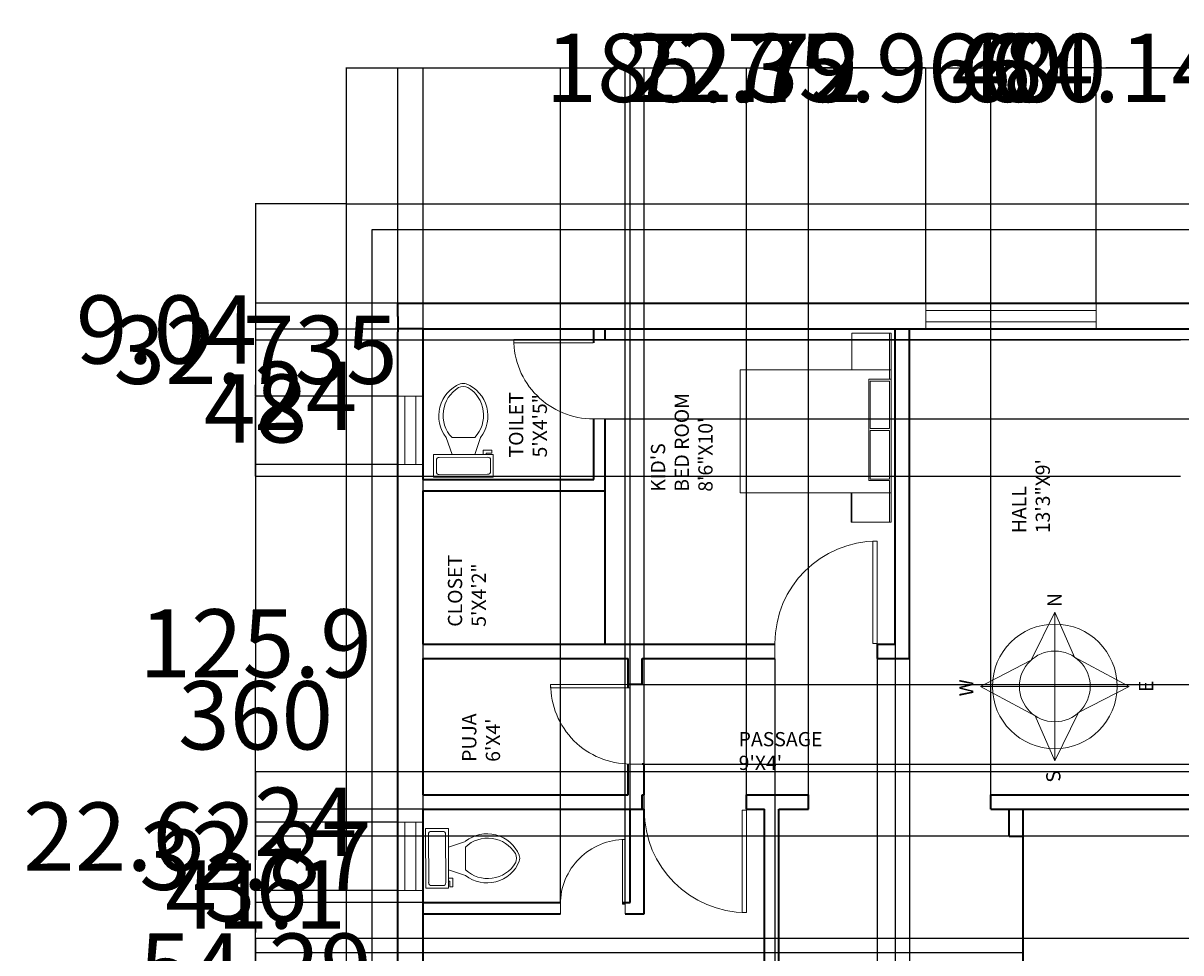
# Model space of a CAD drawing. Units: inches. Extents: x -1643 to -931, y 1907 to 2415.
# Tile 2 of 3: x -1643 to -1236, y 2088 to 2415. Entities that reach past the tile are written whole.
import ezdxf

# ---------------------------------------------------------------- set-up
doc = ezdxf.new("R2010")
doc.units = ezdxf.units.IN
for name, color, linetype, lineweight in [('A-ANNO-DIMS', 2, 'Continuous', 18), ('A-ANNO-SYMB', 7, 'Continuous', 18), ('A-AREA-IDEN', 7, 'Continuous', 18), ('A-DOOR', 3, 'Continuous', 18), ('A-FLOR-FIXT', 9, 'Continuous', 18), ('A-FURN', 8, 'Continuous', 18), ('A-GLAZ', 4, 'Continuous', 18), ('A-WALL', 7, 'Continuous', 35), ('C-PROP', 8, 'Continuous', 25)]:
    doc.layers.add(name, color=color, linetype=linetype, lineweight=lineweight)
doc.styles.get("Standard").update_dxf_attribs({"font": 'arial.ttf', "height": 24})
doc.dimstyles.get("Standard").update_dxf_attribs({"dimtxt": 0.18, "dimasz": 0.18, "dimexe": 0.18, "dimexo": 0.0625, "dimgap": 0.09, "dimtad": 0, "dimtih": 1, "dimtoh": 1, "dimdec": 4, "dimzin": 0, "dimdsep": 46, "dimtxsty": 'Standard', "dimcen": 0.09, "dimadec": 0, "dimazin": 0, "dimtfac": 1, "dimtdec": 4, "dimtofl": 0, "dimtmove": 0, "dimatfit": 3, "dimfxl": 1, "dimtolj": 1, "dimtzin": 0, "dimarcsym": 0})

# ---------------------------------------------------------------- blocks, each defined once
blk = doc.blocks.new('*U2')
for p, q in [((-40, 0), (-40, 6)), ((0, 0), (0, 6))]:
    blk.add_line(p, q)
blk.add_lwpolyline([(0, 0), (0, -40), (-1.75, -40), (-1.75, 0)], close=True)
blk.add_arc((0, 0), 40, 180, 270)
blk = doc.blocks.new('*U6')
for p, q in [((0, 0), (0, -6)), ((-40, 0), (-40, -6))]:
    blk.add_line(p, q)
blk.add_lwpolyline([(0, 0), (0, 40), (-1.75, 40), (-1.75, 0)], close=True)
blk.add_arc((0, 0), 40, 90, 180)
blk = doc.blocks.new('*U5')
for p, q in [((0, 0), (0, 6)), ((40, 0), (40, 6))]:
    blk.add_line(p, q)
blk.add_lwpolyline([(0, 0), (0, -40), (1.75, -40), (1.75, 0)], close=True)
blk.add_arc((0, 0), 40, 270, 0)
blk = doc.blocks.new('*U7')
for p, q in [((0, 5), (0, 0)), ((24, 5), (24, 0)), ((0, 2.5), (24, 2.5))]:
    blk.add_line(p, q)
blk = doc.blocks.new('*U10')
for p, q in [((0, 5), (0, 0)), ((60, 5), (60, 0)), ((0, 2.5), (60, 2.5))]:
    blk.add_line(p, q)
blk = doc.blocks.new('*U9')
for p, q in [((0, 5), (0, 0)), ((60, 5), (60, 0)), ((0, 2.5), (60, 2.5))]:
    blk.add_line(p, q)
blk = doc.blocks.new('*U15')
for p, q in [((-242, 177), (-242, 254)), ((-242, 254), (-216, 254)), ((-216, 254), (-216, 203)), ((-203, 101), (-356, 152)), ((-204, 177), (-242, 177)), ((-216, 203), (-204, 203)), ((-355, -102), (-356, 101)), ((-203, -102), (-355, -153)), ((-152, -242), (-50, -241))]:
    blk.add_line(p, q)
blk.add_lwpolyline([(-203, -267), (1, -267), (-1, 267), (-204, 266)], close=True)
for points in [[(-178, 216), (-177, -216)], [(-51, 241), (-153, 241)], [(-25, -216), (-26, 216)]]:
    blk.add_lwpolyline(points)
for centre, radius, start, end in [((-548, -90), 309, 51.5766, 158.079), ((-156, 219), 22.5, 81.9774, 188.2376), ((-48, 219), 22.5, 351.9774, 98.2376), ((-554, -108), 288, 46.4753, 149.0544), ((-737, -1), 102, 164.9681, 195.247), ((-708, -1), 102, 155.8394, 204.3757), ((-548, 88), 309, 202.136, 308.6382), ((-554, 106), 288, 211.1605, 313.7396), ((-155, -219), 22.5, 171.9774, 278.2376), ((-47, -219), 22.5, 261.9774, 8.2376)]:
    blk.add_arc(centre, radius, start, end)
blk = doc.blocks.new('BED-WITH-NIGHTSTANDS')
for p, q in [((10.33, 53.09), (53.66, 53.09)), ((10.33, 0.09), (10.33, 53.09)), ((53.66, 0.09), (53.66, 53.09)), ((0, 0), (0, 14.11)), ((0, 14.11), (10.33, 14.11)), ((0, 13.84), (10.33, 13.84)), ((53.66, 13.84), (66.5, 13.84)), ((66.5, 0.09), (66.5, 13.84)), ((14.66, 7.89), (50.39, 7.89)), ((14.66, 0.59), (14.66, 7.89)), ((15.11, 7.37), (32.28, 7.37)), ((15.11, 0.59), (15.11, 7.37)), ((32.28, 0.59), (32.28, 7.37)), ((33.01, 0.59), (33.01, 7.37)), ((33.01, 7.37), (49.65, 7.37)), ((49.65, 0.59), (49.65, 7.37)), ((50.39, 0.09), (50.39, 7.89)), ((0, 0.59), (14.66, 0.59)), ((0, 0.09), (66.5, 0.09)), ((15.11, 0.59), (32.28, 0.59)), ((33.01, 0.59), (49.65, 0.59)), ((50.39, 0.59), (66.5, 0.59))]:
    blk.add_line(p, q)
blk = doc.blocks.new('*D21')
at = {"layer": 'A-ANNO-DIMS', "color": 0, "lineweight": -2, "transparency": 16777216}
for p, q in [((-1529.17, 2351.21), (-1529.17, 2399.16)), ((-1528.99, 2398.98), (-1316.21, 2398.98)), ((-1049.35, 2398.98), (-1262.12, 2398.98)), ((-1049.17, 2351.21), (-1049.17, 2399.16))]:
    blk.add_line(p, q, dxfattribs=at)
at = {"layer": 'A-ANNO-DIMS', "color": 0, "transparency": 16777216}
for points in [[(-1528.99, 2399.01), (-1528.99, 2398.95), (-1529.17, 2398.98)], [(-1049.35, 2399.01), (-1049.35, 2398.95), (-1049.17, 2398.98)]]:
    blk.add_solid(points, dxfattribs=at)
at = {"layer": 'Defpoints', "color": 0, "transparency": 16777216}
for p in [(-1049.17, 2398.98), (-1529.17, 2351.15), (-1049.17, 2351.15)]:
    blk.add_point(p, dxfattribs=at)
at = {"layer": 'A-ANNO-DIMS', "color": 0, "transparency": 16777216, "insert": (-1289.17, 2398.98), "char_height": 24, "attachment_point": 5}
blk.add_mtext('\\A1;480', dxfattribs=at)
blk = doc.blocks.new('*D22')
at = {"layer": 'A-ANNO-DIMS', "color": 0, "lineweight": -2, "transparency": 16777216}
for p, q in [((-1529.23, 2351.15), (-1561.32, 2351.15)), ((-1561.14, 2350.97), (-1561.14, 2183.5)), ((-1561.14, 1991.33), (-1561.14, 2158.79)), ((-1529.23, 1991.15), (-1561.32, 1991.15))]:
    blk.add_line(p, q, dxfattribs=at)
at = {"layer": 'A-ANNO-DIMS', "color": 0, "transparency": 16777216}
for points in [[(-1561.17, 2350.97), (-1561.11, 2350.97), (-1561.14, 2351.15)], [(-1561.17, 1991.33), (-1561.11, 1991.33), (-1561.14, 1991.15)]]:
    blk.add_solid(points, dxfattribs=at)
at = {"layer": 'Defpoints', "color": 0, "transparency": 16777216}
for p in [(-1561.14, 2351.15), (-1529.17, 2351.15), (-1529.17, 1991.15)]:
    blk.add_point(p, dxfattribs=at)
at = {"layer": 'A-ANNO-DIMS', "color": 0, "transparency": 16777216, "insert": (-1561.14, 2171.15), "char_height": 24, "attachment_point": 5}
blk.add_mtext('\\A1;360', dxfattribs=at)
blk = doc.blocks.new('*D24')
at = {"layer": 'A-ANNO-DIMS', "color": 0, "lineweight": -2, "transparency": 16777216}
for p, q in [((-1511.17, 2316.21), (-1511.17, 2399.16)), ((-1510.99, 2398.98), (-1457.78, 2398.98)), ((-1325.66, 2398.98), (-1378.87, 2398.98)), ((-1325.48, 2316.19), (-1325.48, 2399.16))]:
    blk.add_line(p, q, dxfattribs=at)
at = {"layer": 'A-ANNO-DIMS', "color": 0, "transparency": 16777216}
for points in [[(-1510.99, 2399.01), (-1510.99, 2398.95), (-1511.17, 2398.98)], [(-1325.66, 2399.01), (-1325.66, 2398.95), (-1325.48, 2398.98)]]:
    blk.add_solid(points, dxfattribs=at)
at = {"layer": 'Defpoints', "color": 0, "transparency": 16777216}
for p in [(-1325.48, 2398.98), (-1511.17, 2316.15), (-1325.48, 2316.13)]:
    blk.add_point(p, dxfattribs=at)
at = {"layer": 'A-ANNO-DIMS', "color": 0, "transparency": 16777216, "insert": (-1418.32, 2398.98), "char_height": 24, "attachment_point": 5}
blk.add_mtext('\\A1;185.7', dxfattribs=at)
blk = doc.blocks.new('*D25')
at = {"layer": 'A-ANNO-DIMS', "color": 0, "lineweight": -2, "transparency": 16777216}
for p, q in [((-1325.48, 2316.19), (-1325.48, 2399.16)), ((-1325.3, 2398.98), (-1312.78, 2398.98)), ((-1265.66, 2398.98), (-1278.17, 2398.98)), ((-1265.48, 2316.19), (-1265.48, 2399.16))]:
    blk.add_line(p, q, dxfattribs=at)
at = {"layer": 'A-ANNO-DIMS', "color": 0, "transparency": 16777216}
for points in [[(-1325.3, 2399.01), (-1325.3, 2398.95), (-1325.48, 2398.98)], [(-1265.66, 2399.01), (-1265.66, 2398.95), (-1265.48, 2398.98)]]:
    blk.add_solid(points, dxfattribs=at)
at = {"layer": 'Defpoints', "color": 0, "transparency": 16777216}
for p in [(-1265.48, 2398.98), (-1325.48, 2316.13), (-1265.48, 2316.13)]:
    blk.add_point(p, dxfattribs=at)
at = {"layer": 'A-ANNO-DIMS', "color": 0, "transparency": 16777216, "insert": (-1295.48, 2398.98), "char_height": 24, "attachment_point": 5}
blk.add_mtext('\\A1;60', dxfattribs=at)
blk = doc.blocks.new('*D26')
at = {"layer": 'A-ANNO-DIMS', "color": 0, "lineweight": -2, "transparency": 16777216}
for p, q in [((-1265.48, 2316.19), (-1265.48, 2399.16)), ((-1265.3, 2398.98), (-1208.35, 2398.98)), ((-1208.17, 2316.21), (-1208.17, 2399.16)), ((-1208.17, 2398.98), (-1207.99, 2398.98))]:
    blk.add_line(p, q, dxfattribs=at)
at = {"layer": 'A-ANNO-DIMS', "color": 0, "transparency": 16777216}
for points in [[(-1265.3, 2399.01), (-1265.3, 2398.95), (-1265.48, 2398.98)], [(-1208.35, 2399.01), (-1208.35, 2398.95), (-1208.17, 2398.98)]]:
    blk.add_solid(points, dxfattribs=at)
at = {"layer": 'Defpoints', "color": 0, "transparency": 16777216}
for p in [(-1208.17, 2398.98), (-1265.48, 2316.13), (-1208.17, 2316.15)]:
    blk.add_point(p, dxfattribs=at)
at = {"layer": 'A-ANNO-DIMS', "color": 0, "transparency": 16777216, "insert": (-1169.72, 2398.98), "char_height": 24, "attachment_point": 5}
blk.add_mtext('\\A1;57.31', dxfattribs=at)
blk = doc.blocks.new('*D33')
at = {"layer": 'A-ANNO-DIMS', "color": 0, "lineweight": -2, "transparency": 16777216}
for p, q in [((-1502.23, 2138.15), (-1561.32, 2138.15)), ((-1561.14, 2137.97), (-1561.14, 2134.06)), ((-1561.14, 2105.46), (-1561.14, 2109.36)), ((-1502.23, 2105.28), (-1561.32, 2105.28))]:
    blk.add_line(p, q, dxfattribs=at)
at = {"layer": 'A-ANNO-DIMS', "color": 0, "transparency": 16777216}
for points in [[(-1561.17, 2137.97), (-1561.11, 2137.97), (-1561.14, 2138.15)], [(-1561.17, 2105.46), (-1561.11, 2105.46), (-1561.14, 2105.28)]]:
    blk.add_solid(points, dxfattribs=at)
at = {"layer": 'Defpoints', "color": 0, "transparency": 16777216}
for p in [(-1502.17, 2138.15), (-1561.14, 2105.28), (-1502.17, 2105.28)]:
    blk.add_point(p, dxfattribs=at)
at = {"layer": 'A-ANNO-DIMS', "color": 0, "transparency": 16777216, "insert": (-1561.14, 2121.71), "char_height": 24, "attachment_point": 5}
blk.add_mtext('\\A1;32.87', dxfattribs=at)
blk = doc.blocks.new('*D34')
at = {"layer": 'A-ANNO-DIMS', "color": 0, "lineweight": -2, "transparency": 16777216}
for p, q in [((-1502.17, 2138.21), (-1502.17, 2399.16)), ((-1501.99, 2398.98), (-1429.63, 2398.98)), ((-1429.45, 2138.21), (-1429.45, 2399.16)), ((-1429.45, 2398.98), (-1429.27, 2398.98))]:
    blk.add_line(p, q, dxfattribs=at)
at = {"layer": 'A-ANNO-DIMS', "color": 0, "transparency": 16777216}
for points in [[(-1501.99, 2399.01), (-1501.99, 2398.95), (-1502.17, 2398.98)], [(-1429.63, 2399.01), (-1429.63, 2398.95), (-1429.45, 2398.98)]]:
    blk.add_solid(points, dxfattribs=at)
at = {"layer": 'Defpoints', "color": 0, "transparency": 16777216}
for p in [(-1429.45, 2398.98), (-1502.17, 2138.15), (-1429.45, 2138.15)]:
    blk.add_point(p, dxfattribs=at)
at = {"layer": 'A-ANNO-DIMS', "color": 0, "transparency": 16777216, "insert": (-1388.91, 2398.98), "char_height": 24, "attachment_point": 5}
blk.add_mtext('\\A1;72.72', dxfattribs=at)
blk = doc.blocks.new('*D41')
at = {"layer": 'A-ANNO-DIMS', "color": 0, "lineweight": -2, "transparency": 16777216}
for p, q in [((-1235.81, 2303.15), (-1561.32, 2303.15)), ((-1561.14, 2302.97), (-1561.14, 2291.5)), ((-1561.14, 2255.33), (-1561.14, 2266.81)), ((-1235.81, 2255.15), (-1561.32, 2255.15))]:
    blk.add_line(p, q, dxfattribs=at)
at = {"layer": 'A-ANNO-DIMS', "color": 0, "transparency": 16777216}
for points in [[(-1561.17, 2302.97), (-1561.11, 2302.97), (-1561.14, 2303.15)], [(-1561.17, 2255.33), (-1561.11, 2255.33), (-1561.14, 2255.15)]]:
    blk.add_solid(points, dxfattribs=at)
at = {"layer": 'Defpoints', "color": 0, "transparency": 16777216}
for p in [(-1235.74, 2303.15), (-1561.14, 2255.15), (-1235.74, 2255.15)]:
    blk.add_point(p, dxfattribs=at)
at = {"layer": 'A-ANNO-DIMS', "color": 0, "transparency": 16777216, "insert": (-1561.14, 2279.15), "char_height": 24, "attachment_point": 5}
blk.add_mtext('\\A1;48', dxfattribs=at)
blk = doc.blocks.new('*D44')
at = {"layer": 'A-ANNO-DIMS', "color": 0, "lineweight": -2, "transparency": 16777216}
for p, q in [((-1213.24, 2151.26), (-1561.32, 2151.26)), ((-1561.14, 2151.08), (-1561.14, 2128.82)), ((-1213.11, 2128.64), (-1561.32, 2128.64)), ((-1561.14, 2128.46), (-1561.32, 2128.46)), ((-1561.14, 2128.64), (-1561.14, 2128.46))]:
    blk.add_line(p, q, dxfattribs=at)
at = {"layer": 'A-ANNO-DIMS', "color": 0, "transparency": 16777216}
for points in [[(-1561.17, 2151.08), (-1561.11, 2151.08), (-1561.14, 2151.26)], [(-1561.17, 2128.82), (-1561.11, 2128.82), (-1561.14, 2128.64)]]:
    blk.add_solid(points, dxfattribs=at)
at = {"layer": 'Defpoints', "color": 0, "transparency": 16777216}
for p in [(-1213.18, 2151.26), (-1561.14, 2128.64), (-1213.05, 2128.64)]:
    blk.add_point(p, dxfattribs=at)
at = {"layer": 'A-ANNO-DIMS', "color": 0, "transparency": 16777216, "insert": (-1601.99, 2128.46), "char_height": 24, "attachment_point": 5}
blk.add_mtext('\\A1;22.62', dxfattribs=at)
blk = doc.blocks.new('*D45')
at = {"layer": 'A-ANNO-DIMS', "color": 0, "lineweight": -2, "transparency": 16777216}
for p, q in [((-1213.11, 2128.64), (-1561.32, 2128.64)), ((-1561.14, 2128.46), (-1561.14, 2122.99)), ((-1561.14, 2092.82), (-1561.14, 2098.29)), ((-1213.11, 2092.64), (-1561.32, 2092.64))]:
    blk.add_line(p, q, dxfattribs=at)
at = {"layer": 'A-ANNO-DIMS', "color": 0, "transparency": 16777216}
for points in [[(-1561.17, 2128.46), (-1561.11, 2128.46), (-1561.14, 2128.64)], [(-1561.17, 2092.82), (-1561.11, 2092.82), (-1561.14, 2092.64)]]:
    blk.add_solid(points, dxfattribs=at)
at = {"layer": 'Defpoints', "color": 0, "transparency": 16777216}
for p in [(-1213.05, 2128.64), (-1561.14, 2092.64), (-1213.05, 2092.64)]:
    blk.add_point(p, dxfattribs=at)
at = {"layer": 'A-ANNO-DIMS', "color": 0, "transparency": 16777216, "insert": (-1561.14, 2110.64), "char_height": 24, "attachment_point": 5}
blk.add_mtext('\\A1;36', dxfattribs=at)
blk = doc.blocks.new('*D46')
at = {"layer": 'A-ANNO-DIMS', "color": 0, "lineweight": -2, "transparency": 16777216}
for p, q in [((-1213.11, 2092.64), (-1561.32, 2092.64)), ((-1561.14, 2092.46), (-1561.14, 2067.69)), ((-1561.14, 2018.33), (-1561.14, 2043.1)), ((-1213.23, 2018.15), (-1561.32, 2018.15))]:
    blk.add_line(p, q, dxfattribs=at)
at = {"layer": 'A-ANNO-DIMS', "color": 0, "transparency": 16777216}
for points in [[(-1561.17, 2092.46), (-1561.11, 2092.46), (-1561.14, 2092.64)], [(-1561.17, 2018.33), (-1561.11, 2018.33), (-1561.14, 2018.15)]]:
    blk.add_solid(points, dxfattribs=at)
at = {"layer": 'Defpoints', "color": 0, "transparency": 16777216}
for p in [(-1213.05, 2092.64), (-1561.14, 2018.15), (-1213.17, 2018.15)]:
    blk.add_point(p, dxfattribs=at)
at = {"layer": 'A-ANNO-DIMS', "color": 0, "transparency": 16777216, "insert": (-1561.14, 2055.39), "char_height": 24, "attachment_point": 5}
blk.add_mtext('\\A1;74.5', dxfattribs=at)
blk = doc.blocks.new('*D49')
at = {"layer": 'A-ANNO-DIMS', "color": 0, "lineweight": -2, "transparency": 16777216}
for p, q in [((-1511.21, 2109.52), (-1561.32, 2109.52)), ((-1561.14, 2109.34), (-1561.14, 2094.71)), ((-1561.14, 2055.4), (-1561.14, 2070.03)), ((-1511.27, 2055.22), (-1561.32, 2055.22))]:
    blk.add_line(p, q, dxfattribs=at)
at = {"layer": 'A-ANNO-DIMS', "color": 0, "transparency": 16777216}
for points in [[(-1561.17, 2109.34), (-1561.11, 2109.34), (-1561.14, 2109.52)], [(-1561.17, 2055.4), (-1561.11, 2055.4), (-1561.14, 2055.22)]]:
    blk.add_solid(points, dxfattribs=at)
at = {"layer": 'Defpoints', "color": 0, "transparency": 16777216}
for p in [(-1561.14, 2109.52), (-1511.15, 2109.52), (-1511.21, 2055.22)]:
    blk.add_point(p, dxfattribs=at)
at = {"layer": 'A-ANNO-DIMS', "color": 0, "transparency": 16777216, "insert": (-1561.14, 2082.37), "char_height": 24, "attachment_point": 5}
blk.add_mtext('\\A1;54.29', dxfattribs=at)
blk = doc.blocks.new('*D50')
at = {"layer": 'A-ANNO-DIMS', "color": 0, "lineweight": -2, "transparency": 16777216}
for p, q in [((-1511.21, 2133.52), (-1561.32, 2133.52)), ((-1561.14, 2133.52), (-1561.14, 2133.7)), ((-1561.14, 2133.7), (-1560.96, 2133.7)), ((-1561.14, 2109.7), (-1561.14, 2133.34)), ((-1511.21, 2109.52), (-1561.32, 2109.52))]:
    blk.add_line(p, q, dxfattribs=at)
at = {"layer": 'A-ANNO-DIMS', "color": 0, "transparency": 16777216}
for points in [[(-1561.17, 2133.34), (-1561.11, 2133.34), (-1561.14, 2133.52)], [(-1561.17, 2109.7), (-1561.11, 2109.7), (-1561.14, 2109.52)]]:
    blk.add_solid(points, dxfattribs=at)
at = {"layer": 'Defpoints', "color": 0, "transparency": 16777216}
for p in [(-1561.14, 2133.52), (-1511.15, 2133.52), (-1511.15, 2109.52)]:
    blk.add_point(p, dxfattribs=at)
at = {"layer": 'A-ANNO-DIMS', "color": 0, "transparency": 16777216, "insert": (-1543.53, 2133.7), "char_height": 24, "attachment_point": 5}
blk.add_mtext('\\A1;24', dxfattribs=at)
blk = doc.blocks.new('*D51')
at = {"layer": 'A-ANNO-DIMS', "color": 0, "lineweight": -2, "transparency": 16777216}
for p, q in [((-1511.22, 2259.41), (-1561.32, 2259.41)), ((-1561.14, 2259.23), (-1561.14, 2208.81)), ((-1561.14, 2133.7), (-1561.14, 2184.12)), ((-1511.21, 2133.52), (-1561.32, 2133.52))]:
    blk.add_line(p, q, dxfattribs=at)
at = {"layer": 'A-ANNO-DIMS', "color": 0, "transparency": 16777216}
for points in [[(-1561.17, 2259.23), (-1561.11, 2259.23), (-1561.14, 2259.41)], [(-1561.17, 2133.7), (-1561.11, 2133.7), (-1561.14, 2133.52)]]:
    blk.add_solid(points, dxfattribs=at)
at = {"layer": 'Defpoints', "color": 0, "transparency": 16777216}
for p in [(-1561.14, 2259.41), (-1511.16, 2259.41), (-1511.15, 2133.52)]:
    blk.add_point(p, dxfattribs=at)
at = {"layer": 'A-ANNO-DIMS', "color": 0, "transparency": 16777216, "insert": (-1561.14, 2196.46), "char_height": 24, "attachment_point": 5}
blk.add_mtext('\\A1;125.9', dxfattribs=at)
blk = doc.blocks.new('*D52')
at = {"layer": 'A-ANNO-DIMS', "color": 0, "lineweight": -2, "transparency": 16777216}
for p, q in [((-1511.22, 2283.41), (-1561.32, 2283.41)), ((-1561.14, 2283.41), (-1561.14, 2283.59)), ((-1561.14, 2283.59), (-1560.96, 2283.59)), ((-1561.14, 2259.59), (-1561.14, 2283.23)), ((-1511.22, 2259.41), (-1561.32, 2259.41))]:
    blk.add_line(p, q, dxfattribs=at)
at = {"layer": 'A-ANNO-DIMS', "color": 0, "transparency": 16777216}
for points in [[(-1561.17, 2283.23), (-1561.11, 2283.23), (-1561.14, 2283.41)], [(-1561.17, 2259.59), (-1561.11, 2259.59), (-1561.14, 2259.41)]]:
    blk.add_solid(points, dxfattribs=at)
at = {"layer": 'Defpoints', "color": 0, "transparency": 16777216}
for p in [(-1561.14, 2283.41), (-1511.16, 2283.41), (-1511.16, 2259.41)]:
    blk.add_point(p, dxfattribs=at)
at = {"layer": 'A-ANNO-DIMS', "color": 0, "transparency": 16777216, "insert": (-1543.53, 2283.59), "char_height": 24, "attachment_point": 5}
blk.add_mtext('\\A1;24', dxfattribs=at)
blk = doc.blocks.new('*D53')
at = {"layer": 'A-ANNO-DIMS', "color": 0, "lineweight": -2, "transparency": 16777216}
for p, q in [((-1511.23, 2316.15), (-1561.32, 2316.15)), ((-1561.14, 2315.97), (-1561.14, 2312.13)), ((-1561.14, 2283.59), (-1561.14, 2287.43)), ((-1511.22, 2283.41), (-1561.32, 2283.41))]:
    blk.add_line(p, q, dxfattribs=at)
at = {"layer": 'A-ANNO-DIMS', "color": 0, "transparency": 16777216}
for points in [[(-1561.17, 2315.97), (-1561.11, 2315.97), (-1561.14, 2316.15)], [(-1561.17, 2283.59), (-1561.11, 2283.59), (-1561.14, 2283.41)]]:
    blk.add_solid(points, dxfattribs=at)
at = {"layer": 'Defpoints', "color": 0, "transparency": 16777216}
for p in [(-1561.14, 2316.15), (-1511.17, 2316.15), (-1511.16, 2283.41)]:
    blk.add_point(p, dxfattribs=at)
at = {"layer": 'A-ANNO-DIMS', "color": 0, "transparency": 16777216, "insert": (-1561.14, 2299.78), "char_height": 24, "attachment_point": 5}
blk.add_mtext('\\A1;32.735', dxfattribs=at)
blk = doc.blocks.new('*D54')
at = {"layer": 'A-ANNO-DIMS', "color": 0, "lineweight": -2, "transparency": 16777216}
for p, q in [((-1438.11, 2303.44), (-971.69, 2303.44)), ((-971.87, 2303.26), (-971.87, 2301.79)), ((-971.87, 2275.62), (-971.87, 2277.1)), ((-1438.11, 2275.44), (-971.69, 2275.44))]:
    blk.add_line(p, q, dxfattribs=at)
at = {"layer": 'A-ANNO-DIMS', "color": 0, "transparency": 16777216}
for points in [[(-971.9, 2303.26), (-971.84, 2303.26), (-971.87, 2303.44)], [(-971.9, 2275.62), (-971.84, 2275.62), (-971.87, 2275.44)]]:
    blk.add_solid(points, dxfattribs=at)
at = {"layer": 'Defpoints', "color": 0, "transparency": 16777216}
for p in [(-1438.17, 2303.44), (-1438.17, 2275.44), (-971.87, 2275.44)]:
    blk.add_point(p, dxfattribs=at)
at = {"layer": 'A-ANNO-DIMS', "color": 0, "transparency": 16777216, "insert": (-971.87, 2289.44), "char_height": 24, "attachment_point": 5}
blk.add_mtext('\\A1;28', dxfattribs=at)
blk = doc.blocks.new('*D55')
at = {"layer": 'A-ANNO-DIMS', "color": 0, "lineweight": -2, "transparency": 16777216}
for p, q in [((-1378.5, 2191.08), (-1378.5, 1922.66)), ((-1342.5, 2191.08), (-1342.5, 1922.66)), ((-1378.32, 1922.84), (-1377.76, 1922.84)), ((-1342.68, 1922.84), (-1343.23, 1922.84))]:
    blk.add_line(p, q, dxfattribs=at)
at = {"layer": 'A-ANNO-DIMS', "color": 0, "transparency": 16777216}
for points in [[(-1378.32, 1922.87), (-1378.32, 1922.81), (-1378.5, 1922.84)], [(-1342.68, 1922.87), (-1342.68, 1922.81), (-1342.5, 1922.84)]]:
    blk.add_solid(points, dxfattribs=at)
at = {"layer": 'Defpoints', "color": 0, "transparency": 16777216}
for p in [(-1378.5, 2191.15), (-1342.5, 2191.15), (-1342.5, 1922.84)]:
    blk.add_point(p, dxfattribs=at)
at = {"layer": 'A-ANNO-DIMS', "color": 0, "transparency": 16777216, "insert": (-1360.5, 1922.84), "char_height": 24, "attachment_point": 5}
blk.add_mtext('\\A1;36', dxfattribs=at)
blk = doc.blocks.new('*D56')
at = {"layer": 'A-ANNO-DIMS', "color": 0, "lineweight": -2, "transparency": 16777216}
for p, q in [((-1425.11, 2182), (-971.69, 2182)), ((-971.87, 2181.82), (-971.87, 2180.35)), ((-1424.39, 2154), (-971.69, 2154)), ((-971.87, 2154.18), (-971.87, 2155.66))]:
    blk.add_line(p, q, dxfattribs=at)
at = {"layer": 'A-ANNO-DIMS', "color": 0, "transparency": 16777216}
for points in [[(-971.9, 2181.82), (-971.84, 2181.82), (-971.87, 2182)], [(-971.9, 2154.18), (-971.84, 2154.18), (-971.87, 2154)]]:
    blk.add_solid(points, dxfattribs=at)
at = {"layer": 'Defpoints', "color": 0, "transparency": 16777216}
for p in [(-1425.17, 2182), (-1424.45, 2154), (-971.87, 2154)]:
    blk.add_point(p, dxfattribs=at)
at = {"layer": 'A-ANNO-DIMS', "color": 0, "transparency": 16777216, "insert": (-971.87, 2168), "char_height": 24, "attachment_point": 5}
blk.add_mtext('\\A1;28', dxfattribs=at)
blk = doc.blocks.new('*D57')
at = {"layer": 'A-ANNO-DIMS', "color": 0, "lineweight": -2, "transparency": 16777216}
for p, q in [((-1424.45, 2138.21), (-1424.45, 2399.16)), ((-1424.27, 2398.98), (-1388.66, 2398.98)), ((-1388.48, 2138.21), (-1388.48, 2399.16)), ((-1388.48, 2398.98), (-1388.3, 2398.98))]:
    blk.add_line(p, q, dxfattribs=at)
at = {"layer": 'A-ANNO-DIMS', "color": 0, "transparency": 16777216}
for points in [[(-1424.27, 2399.01), (-1424.27, 2398.95), (-1424.45, 2398.98)], [(-1388.66, 2399.01), (-1388.66, 2398.95), (-1388.48, 2398.98)]]:
    blk.add_solid(points, dxfattribs=at)
at = {"layer": 'Defpoints', "color": 0, "transparency": 16777216}
for p in [(-1388.48, 2398.98), (-1424.45, 2138.15), (-1388.48, 2138.15)]:
    blk.add_point(p, dxfattribs=at)
at = {"layer": 'A-ANNO-DIMS', "color": 0, "transparency": 16777216, "insert": (-1338.41, 2398.98), "char_height": 24, "attachment_point": 5}
blk.add_mtext('\\A1;35.966', dxfattribs=at)
blk = doc.blocks.new('*D58')
at = {"layer": 'A-ANNO-DIMS', "color": 0, "lineweight": -2, "transparency": 16777216}
for p, q in [((-1453.94, 2105.34), (-1453.94, 2399.16)), ((-1453.76, 2398.98), (-1431.33, 2398.98)), ((-1431.15, 2104.72), (-1431.15, 2399.16)), ((-1431.15, 2398.98), (-1430.97, 2398.98))]:
    blk.add_line(p, q, dxfattribs=at)
at = {"layer": 'A-ANNO-DIMS', "color": 0, "transparency": 16777216}
for points in [[(-1453.76, 2399.01), (-1453.76, 2398.95), (-1453.94, 2398.98)], [(-1431.33, 2399.01), (-1431.33, 2398.95), (-1431.15, 2398.98)]]:
    blk.add_solid(points, dxfattribs=at)
at = {"layer": 'Defpoints', "color": 0, "transparency": 16777216}
for p in [(-1431.15, 2398.98), (-1453.94, 2105.28), (-1431.15, 2104.65)]:
    blk.add_point(p, dxfattribs=at)
at = {"layer": 'A-ANNO-DIMS', "color": 0, "transparency": 16777216, "insert": (-1390.16, 2398.98), "char_height": 24, "attachment_point": 5}
blk.add_mtext('\\A1;22.79', dxfattribs=at)
blk = doc.blocks.new('*D59')
at = {"layer": 'A-ANNO-DIMS', "color": 0, "lineweight": -2, "transparency": 16777216}
for p, q in [((-1366.66, 2143.21), (-1366.66, 2399.16)), ((-1366.48, 2398.98), (-1302.71, 2398.98)), ((-1302.53, 2143.21), (-1302.53, 2399.16)), ((-1302.53, 2398.98), (-1302.35, 2398.98))]:
    blk.add_line(p, q, dxfattribs=at)
at = {"layer": 'A-ANNO-DIMS', "color": 0, "transparency": 16777216}
for points in [[(-1366.48, 2399.01), (-1366.48, 2398.95), (-1366.66, 2398.98)], [(-1302.71, 2399.01), (-1302.71, 2398.95), (-1302.53, 2398.98)]]:
    blk.add_solid(points, dxfattribs=at)
at = {"layer": 'Defpoints', "color": 0, "transparency": 16777216}
for p in [(-1302.53, 2398.98), (-1366.66, 2143.15), (-1302.53, 2143.15)]:
    blk.add_point(p, dxfattribs=at)
at = {"layer": 'A-ANNO-DIMS', "color": 0, "transparency": 16777216, "insert": (-1261.75, 2398.98), "char_height": 24, "attachment_point": 5}
blk.add_mtext('\\A1;64.14', dxfattribs=at)
blk = doc.blocks.new('*D60')
at = {"layer": 'A-ANNO-DIMS', "color": 0, "lineweight": -2, "transparency": 16777216}
for p, q in [((-1291.23, 2128.66), (-1561.32, 2128.66)), ((-1561.14, 2128.48), (-1561.14, 2120.24)), ((-1561.14, 2087.74), (-1561.14, 2095.97)), ((-1291.23, 2087.56), (-1561.32, 2087.56))]:
    blk.add_line(p, q, dxfattribs=at)
at = {"layer": 'A-ANNO-DIMS', "color": 0, "transparency": 16777216}
for points in [[(-1561.17, 2128.48), (-1561.11, 2128.48), (-1561.14, 2128.66)], [(-1561.17, 2087.74), (-1561.11, 2087.74), (-1561.14, 2087.56)]]:
    blk.add_solid(points, dxfattribs=at)
at = {"layer": 'Defpoints', "color": 0, "transparency": 16777216}
for p in [(-1561.14, 2128.66), (-1291.17, 2128.66), (-1291.17, 2087.56)]:
    blk.add_point(p, dxfattribs=at)
at = {"layer": 'A-ANNO-DIMS', "color": 0, "transparency": 16777216, "insert": (-1561.14, 2108.11), "char_height": 24, "attachment_point": 5}
blk.add_mtext('\\A1;41.1', dxfattribs=at)
blk = doc.blocks.new('*D61')
at = {"layer": 'A-ANNO-DIMS', "color": 0, "lineweight": -2, "transparency": 16777216}
for p, q in [((-1325.54, 2316.13), (-1561.32, 2316.13)), ((-1561.14, 2315.95), (-1561.14, 2307.27)), ((-1325.54, 2307.09), (-1561.32, 2307.09)), ((-1561.14, 2306.91), (-1561.32, 2306.91)), ((-1561.14, 2307.09), (-1561.14, 2306.91))]:
    blk.add_line(p, q, dxfattribs=at)
at = {"layer": 'A-ANNO-DIMS', "color": 0, "transparency": 16777216}
for points in [[(-1561.17, 2315.95), (-1561.11, 2315.95), (-1561.14, 2316.13)], [(-1561.17, 2307.27), (-1561.11, 2307.27), (-1561.14, 2307.09)]]:
    blk.add_solid(points, dxfattribs=at)
at = {"layer": 'Defpoints', "color": 0, "transparency": 16777216}
for p in [(-1325.48, 2316.13), (-1561.14, 2307.09), (-1325.48, 2307.09)]:
    blk.add_point(p, dxfattribs=at)
at = {"layer": 'A-ANNO-DIMS', "color": 0, "transparency": 16777216, "insert": (-1592.53, 2306.91), "char_height": 24, "attachment_point": 5}
blk.add_mtext('\\A1;9.04', dxfattribs=at)
blk = doc.blocks.new('*D62')
at = {"layer": 'A-ANNO-DIMS', "color": 0, "lineweight": -2, "transparency": 16777216}
for p, q in [((-1336.17, 2196.08), (-1336.17, 1922.66)), ((-1331.15, 2191.08), (-1331.15, 1922.66)), ((-1335.99, 1922.84), (-1331.33, 1922.84)), ((-1331.15, 1922.84), (-1330.97, 1922.84))]:
    blk.add_line(p, q, dxfattribs=at)
at = {"layer": 'A-ANNO-DIMS', "color": 0, "transparency": 16777216}
for points in [[(-1335.99, 1922.87), (-1335.99, 1922.81), (-1336.17, 1922.84)], [(-1331.33, 1922.87), (-1331.33, 1922.81), (-1331.15, 1922.84)]]:
    blk.add_solid(points, dxfattribs=at)
at = {"layer": 'Defpoints', "color": 0, "transparency": 16777216}
for p in [(-1336.17, 2196.15), (-1331.15, 2191.15), (-1331.15, 1922.84)]:
    blk.add_point(p, dxfattribs=at)
at = {"layer": 'A-ANNO-DIMS', "color": 0, "transparency": 16777216, "insert": (-1290.39, 1922.84), "char_height": 24, "attachment_point": 5}
blk.add_mtext('\\A1;5.013', dxfattribs=at)

msp = doc.modelspace()

# ---------------------------------------------------------------- linework, layer by layer
at = {"layer": 'A-ANNO-SYMB'}
for p, q in [((-1288.4285, 2190.5496), (-1280.072, 2207.4636)), ((-1280.072, 2207.4636), (-1273.1474, 2191.6673)), ((-1280.072, 2155.1759), (-1280.072, 2207.4636)), ((-1288.4285, 2190.5496), (-1306.2158, 2181.3197)), ((-1253.9281, 2181.3197), (-1273.1474, 2191.6673)), ((-1306.2158, 2181.3197), (-1286.9965, 2170.9721)), ((-1306.2158, 2181.3197), (-1253.9281, 2181.3197)), ((-1280.072, 2181.3197), (-1280.072, 2181.3197)), ((-1271.7154, 2172.0899), (-1253.9281, 2181.3197)), ((-1286.9965, 2170.9721), (-1280.072, 2155.1759)), ((-1280.072, 2155.1759), (-1271.7154, 2172.0899))]:
    msp.add_line(p, q, dxfattribs=at)
for radius in [21.9386, 12.4508]:
    msp.add_circle((-1280.072, 2181.3197), radius, dxfattribs=at)
at = {"layer": 'A-WALL'}
for p, q in [((-1511.1668, 2316.1464), (-1131.1668, 2316.1464)), ((-1511.1668, 2311.4873), (-1511.1668, 2316.1464)), ((-1511.1668, 2311.4873), (-1511.1668, 2306.1464)), ((-1502.1668, 2307.1464), (-1511.1668, 2307.1464)), ((-1511.1668, 2009.1464), (-1511.1668, 2306.1464)), ((-1502.1668, 2306.1464), (-1502.1668, 2307.1464)), ((-1502.1668, 2307.1464), (-1213.1668, 2307.1464)), ((-1502.1668, 2254.1464), (-1502.1668, 2306.1464)), ((-1442.1668, 2306.1464), (-1442.1668, 2307.1464)), ((-1442.1668, 2302.2175), (-1442.1668, 2306.1464)), ((-1438.1668, 2306.1464), (-1438.1668, 2307.1464)), ((-1438.1668, 2303.4425), (-1438.1668, 2306.1464)), ((-1336.1668, 2306.1464), (-1336.1668, 2307.1464)), ((-1336.1668, 2196.1464), (-1336.1668, 2306.1464)), ((-1331.1668, 2306.1464), (-1331.1668, 2307.1464)), ((-1331.1668, 2196.1464), (-1331.1668, 2306.1464)), ((-1442.1668, 2254.1464), (-1442.1668, 2275.4654)), ((-1438.1668, 2196.1464), (-1438.1668, 2275.4425)), ((-1502.1668, 2254.1464), (-1442.1668, 2254.1464)), ((-1502.1668, 2250.1464), (-1438.1668, 2250.1464)), ((-1502.1668, 2196.1464), (-1502.1668, 2250.1464)), ((-1502.1668, 2196.1464), (-1378.4982, 2196.1464)), ((-1342.4982, 2196.1464), (-1336.1668, 2196.1464)), ((-1342.4982, 2196.1464), (-1342.4982, 2191.1464)), ((-1331.1542, 2191.1464), (-1331.1668, 2196.1464)), ((-1502.1668, 2191.1464), (-1430.1668, 2191.1464)), ((-1502.1668, 2143.1464), (-1502.1668, 2191.1464)), ((-1430.1668, 2180.7784), (-1430.1668, 2191.1464)), ((-1425.1668, 2191.1464), (-1378.4982, 2191.1464)), ((-1425.1668, 2182.1464), (-1425.1668, 2191.1464)), ((-1342.4982, 2191.1464), (-1331.1542, 2191.1464)), ((-1430.1668, 2182.1464), (-1425.1668, 2182.1464)), ((-1430.1668, 2143.1464), (-1430.1668, 2154.0147)), ((-1424.4498, 2154.0034), (-1425.1708, 2154.0034)), ((-1424.4498, 2143.1464), (-1424.4498, 2154.0034)), ((-1502.1668, 2143.1464), (-1430.1668, 2143.1464)), ((-1425.1668, 2138.1464), (-1425.1668, 2143.1464)), ((-1425.1668, 2143.1464), (-1424.4498, 2143.1464)), ((-1388.4842, 2138.1464), (-1388.4842, 2143.1464)), ((-1388.4842, 2143.1464), (-1382.1668, 2143.1464)), ((-1382.1668, 2143.1464), (-1366.6634, 2143.1464)), ((-1366.6634, 2138.1464), (-1366.6634, 2143.1464)), ((-1302.5278, 2143.1464), (-1213.1668, 2143.1464)), ((-1302.5278, 2138.1464), (-1302.5278, 2143.1464)), ((-1502.1668, 2018.1464), (-1502.1668, 2138.1464)), ((-1502.1668, 2138.1464), (-1425.1668, 2138.1464)), ((-1429.4498, 2105.2782), (-1429.4498, 2138.1464)), ((-1425.1668, 2138.1464), (-1424.4498, 2138.1464)), ((-1424.4498, 2101.2782), (-1424.4498, 2138.1464)), ((-1388.4842, 2138.1464), (-1382.1668, 2138.1464)), ((-1382.1668, 2018.1464), (-1382.1668, 2138.1464)), ((-1377.1668, 2018.1464), (-1377.1668, 2138.1464)), ((-1377.1668, 2138.1464), (-1366.6634, 2138.1464)), ((-1302.5278, 2138.1464), (-1296.1668, 2138.1464)), ((-1296.1668, 2138.1464), (-1291.1668, 2138.1464)), ((-1296.1668, 2138.1464), (-1291.1668, 2138.1464)), ((-1296.1668, 2128.6553), (-1296.1668, 2138.1464)), ((-1291.1668, 2018.1464), (-1291.1668, 2138.1464)), ((-1291.1668, 2138.1464), (-1213.1668, 2138.1464)), ((-1296.1668, 2128.6553), (-1291.1668, 2128.6553)), ((-1502.1668, 2105.2782), (-1453.9433, 2105.2782)), ((-1432.149, 2105.2782), (-1429.4498, 2105.2782)), ((-1502.1668, 2101.2782), (-1453.9519, 2101.2782)), ((-1431.1514, 2101.2782), (-1425.1668, 2101.2782)), ((-1425.1668, 2101.2782), (-1424.4498, 2101.2782))]:
    msp.add_line(p, q, dxfattribs=at)
at = {"layer": 'C-PROP'}
for p, q in [((-1529.1668, 1991.1464), (-1529.1668, 2351.1464)), ((-1529.1668, 2351.1464), (-1049.1668, 2351.1464)), ((-1520.1668, 2000.1464), (-1520.1668, 2342.1464)), ((-1520.1668, 2342.1464), (-1058.1668, 2342.1464))]:
    msp.add_line(p, q, dxfattribs=at)

# ---------------------------------------------------------------- block references
at = {"layer": 'A-DOOR'}
for p, xscale, yscale, zscale, rotation in [((-1442.3708, 2303.4425), 0.7000000000000001, 0.7000000000000001, 0.7000000000000001, 270), ((-1429.3708, 2182.0034), 0.7000000000000001, 0.7000000000000001, 0.7000000000000001, 270), ((-1431.1514, 2104.6534), 0.5700110980006006, 0.5700110980006006, 0.5700110980006006, 180)]:
    msp.add_blockref('*U5', p, dxfattribs=dict(at, xscale=xscale, yscale=yscale, zscale=zscale, rotation=rotation))
at = {"layer": 'A-DOOR', "xscale": 0.9, "yscale": 0.9, "zscale": 0.9}
for name, p in [('*U6', (-1342.4982, 2196.4667)), ('*U2', (-1388.4498, 2137.7465))]:
    msp.add_blockref(name, p, dxfattribs=at)
at = {"layer": 'A-FLOR-FIXT', "xscale": 0.0393700787401575, "yscale": 0.0393700787401575, "zscale": 0.0393700787401575}
for p, rotation in [((-1488.0437, 2254.9428), 270), ((-1501.2909, 2120.7761), 180)]:
    msp.add_blockref('*U15', p, dxfattribs=dict(at, rotation=rotation))
at = {"layer": 'A-FURN', "rotation": 90.0000000000013}
msp.add_blockref('BED-WITH-NIGHTSTANDS', (-1337.5769, 2239.0844), dxfattribs=at)
at = {"layer": 'A-GLAZ'}
for name, p in [('*U9', (-1325.4771, 2311.1314)), ('*U10', (-1325.478, 2307.092))]:
    msp.add_blockref(name, p, dxfattribs=at)
at = {"layer": 'A-GLAZ', "rotation": 270}
for p in [(-1511.1597, 2283.4112), (-1507.2375, 2283.4165), (-1511.1453, 2133.516), (-1507.2375, 2133.5243)]:
    msp.add_blockref('*U7', p, dxfattribs=at)

# ---------------------------------------------------------------- texts
at = {"layer": 'A-ANNO-SYMB', "char_height": 5, "attachment_point": 1}
for s, width, insert, rotation in [('N', 10.988887, (-1282.6739, 2209.2546), 90), ('W', 48.389659, (-1313.6974, 2177.8217), 90), ('E', 11.952828, (-1250.4755, 2179.3488), 90), ('S', 34.508966, (-1282.7555, 2147.2289), 98.36296)]:
    msp.add_mtext_dynamic_manual_height_columns(s, width=width, gutter_width=120, heights=[0], dxfattribs=dict(at, insert=insert, rotation=rotation))
at = {"layer": 'A-AREA-IDEN', "char_height": 5, "attachment_point": 1, "rotation": 90}
for s, width, insert in [('TOILET\\P5\'X4\'5"', 106.496123, (-1472.0099, 2261.8962)), ('KID\'S\\PBED ROOM\\P8\'6"X10\'', 50.968561, (-1422.0953, 2249.8293)), ('HALL\\P13\'3"X9\'', 56.726574, (-1295.1218, 2235.2391)), ('CLOSET\\P5\'X4\'2"', 73.534199, (-1493.4986, 2202.3169)), ("PUJA\\P6'X4'", 153.656396, (-1488.4992, 2154.7803))]:
    msp.add_mtext_dynamic_manual_height_columns(s, width=width, gutter_width=120, heights=[0], dxfattribs=dict(at, insert=insert))
at = {"layer": 'A-AREA-IDEN', "insert": (-1391.2395, 2165.256), "char_height": 5, "attachment_point": 1}
msp.add_mtext_dynamic_manual_height_columns("PASSAGE\\P9'X4'", width=49.293418, gutter_width=120, heights=[0], dxfattribs=at)

# ---------------------------------------------------------------- dimensions: what is measured, and where the dimension line sits
at = {"layer": 'A-ANNO-DIMS'}
for base, p1, p2, override, picture, middle in [((-1049.1668, 2398.9832), (-1529.1668, 2351.1464), (-1049.1668, 2351.1464), {"dimdec": 0, "dimlfac": 1, "dimrnd": 0, "dimzin": 0, "dimdsep": 46, "dimlunit": 2}, '*D21', (-1289.1668, 2398.9832)), ((-1325.4771, 2398.9832), (-1511.1668, 2316.1464), (-1325.4771, 2316.1314), {"dimdec": 1, "dimlfac": 1, "dimrnd": 0, "dimzin": 0, "dimdsep": 46, "dimlunit": 2}, '*D24', (-1418.322, 2398.9832)), ((-1429.4498, 2398.9832), (-1502.1668, 2138.1464), (-1429.4498, 2138.1464), {"dimdec": 2, "dimlfac": 1, "dimrnd": 0, "dimzin": 0, "dimdsep": 46, "dimlunit": 2}, '*D34', (-1388.9069, 2398.9832)), ((-1431.1514, 2398.9832), (-1453.9433, 2105.2782), (-1431.1514, 2104.6534), {"dimdec": 2, "dimlfac": 1, "dimrnd": 0, "dimzin": 0, "dimdsep": 46, "dimlunit": 2}, '*D58', (-1390.1584, 2398.9832)), ((-1388.4842, 2398.9832), (-1424.4498, 2138.1464), (-1388.4842, 2138.1464), {"dimdec": 3, "dimlfac": 1, "dimrnd": 0, "dimzin": 0, "dimdsep": 46, "dimlunit": 2}, '*D57', (-1338.4134, 2398.9832)), ((-1302.5278, 2398.9832), (-1366.6634, 2143.1464), (-1302.5278, 2143.1464), {"dimdec": 2, "dimlfac": 1, "dimrnd": 0, "dimzin": 0, "dimdsep": 46, "dimlunit": 2}, '*D59', (-1261.7476, 2398.9832)), ((-1265.4771, 2398.9832), (-1325.4771, 2316.1314), (-1265.4771, 2316.1314), {"dimdec": 0, "dimlfac": 1, "dimrnd": 0, "dimzin": 0, "dimdsep": 46, "dimlunit": 2}, '*D25', (-1295.4771, 2398.9832)), ((-1208.1668, 2398.9832), (-1265.4771, 2316.1314), (-1208.1668, 2316.1464), {"dimdec": 2, "dimlfac": 1, "dimrnd": 0, "dimzin": 0, "dimdsep": 46, "dimlunit": 2}, '*D26', (-1169.7195, 2398.9832)), ((-1331.1542, 1922.8359), (-1336.1668, 2196.1464), (-1331.1542, 2191.1464), {"dimdec": 3, "dimlfac": 1, "dimrnd": 0, "dimzin": 0, "dimdsep": 46, "dimlunit": 2}, '*D62', (-1290.3903, 1922.8359)), ((-1342.4982, 1922.8359), (-1378.4982, 2191.1464), (-1342.4982, 2191.1464), {"dimdec": 0, "dimlfac": 1, "dimrnd": 0, "dimzin": 0, "dimdsep": 46, "dimlunit": 2}, '*D55', (-1360.4982, 1922.8359))]:
    dim = msp.add_linear_dim(base=base, p1=p1, p2=p2, dimstyle='Standard', override=override, dxfattribs=at)
    dim.commit()
    dim.dimension.update_dxf_attribs({"geometry": picture, "text_midpoint": middle})
for base, p1, p2, override, picture, middle in [((-1561.1409, 2351.1464), (-1529.1668, 1991.1464), (-1529.1668, 2351.1464), {"dimdec": 0, "dimlfac": 1, "dimrnd": 0, "dimzin": 0, "dimdsep": 46, "dimlunit": 2}, '*D22', (-1561.1409, 2171.1464)), ((-1561.1409, 2307.092), (-1325.4771, 2316.1314), (-1325.478, 2307.092), {"dimdec": 2, "dimlfac": 1, "dimrnd": 0, "dimzin": 0, "dimdsep": 46, "dimlunit": 2}, '*D61', (-1592.5324, 2306.912)), ((-1561.1409, 2316.1464), (-1511.1597, 2283.4112), (-1511.1668, 2316.1464), {"dimdec": 3, "dimlfac": 1, "dimrnd": 0, "dimzin": 0, "dimdsep": 46, "dimlunit": 2}, '*D53', (-1561.1409, 2299.7788)), ((-971.8662, 2275.4425), (-1438.1708, 2303.4425), (-1438.1708, 2275.4425), {"dimdec": 0, "dimlfac": 1, "dimrnd": 0, "dimzin": 0, "dimdsep": 46, "dimlunit": 2}, '*D54', (-971.8662, 2289.4425)), ((-1561.1409, 2255.1527), (-1235.7435, 2303.1527), (-1235.7435, 2255.1527), {"dimdec": 0, "dimlfac": 1, "dimrnd": 0, "dimzin": 0, "dimdsep": 46, "dimlunit": 2}, '*D41', (-1561.1409, 2279.1527)), ((-1561.1409, 2283.4112), (-1511.1597, 2259.4112), (-1511.1597, 2283.4112), {"dimdec": 0, "dimlfac": 1, "dimrnd": 0, "dimzin": 0, "dimdsep": 46, "dimlunit": 2}, '*D52', (-1543.5258, 2283.5912)), ((-1561.1409, 2259.4112), (-1511.1453, 2133.516), (-1511.1597, 2259.4112), {"dimdec": 1, "dimlfac": 1, "dimrnd": 0, "dimzin": 0, "dimdsep": 46, "dimlunit": 2}, '*D51', (-1561.1409, 2196.4636)), ((-971.8662, 2154.0034), (-1425.1708, 2182.0034), (-1424.4498, 2154.0034), {"dimdec": 0, "dimlfac": 1, "dimrnd": 0, "dimzin": 0, "dimdsep": 46, "dimlunit": 2}, '*D56', (-971.8662, 2168.0034)), ((-1561.1409, 2128.64), (-1213.1766, 2151.2595), (-1213.047, 2128.64), {"dimdec": 2, "dimlfac": 1, "dimrnd": 0, "dimzin": 0, "dimdsep": 46, "dimlunit": 2}, '*D44', (-1601.9867, 2128.46)), ((-1561.1409, 2133.516), (-1511.1453, 2109.516), (-1511.1453, 2133.516), {"dimdec": 0, "dimlfac": 1, "dimrnd": 0, "dimzin": 0, "dimdsep": 46, "dimlunit": 2}, '*D50', (-1543.5258, 2133.696)), ((-1561.1409, 2105.2782), (-1502.1668, 2138.1464), (-1502.1668, 2105.2782), {"dimdec": 2, "dimlfac": 1, "dimrnd": 0, "dimzin": 0, "dimdsep": 46, "dimlunit": 2}, '*D33', (-1561.1409, 2121.7123)), ((-1561.1409, 2128.6553), (-1291.1668, 2087.5551), (-1291.1668, 2128.6553), {"dimdec": 1, "dimlfac": 1, "dimrnd": 0, "dimzin": 0, "dimdsep": 46, "dimlunit": 2}, '*D60', (-1561.1409, 2108.1052)), ((-1561.1409, 2092.64), (-1213.047, 2128.64), (-1213.047, 2092.64), {"dimdec": 0, "dimlfac": 1, "dimrnd": 0, "dimzin": 0, "dimdsep": 46, "dimlunit": 2}, '*D45', (-1561.1409, 2110.64)), ((-1561.1409, 2109.516), (-1511.2115, 2055.2238), (-1511.1453, 2109.516), {"dimdec": 2, "dimlfac": 1, "dimrnd": 0, "dimzin": 0, "dimdsep": 46, "dimlunit": 2}, '*D49', (-1561.1409, 2082.3699)), ((-1561.1409, 2018.1464), (-1213.047, 2092.64), (-1213.1668, 2018.1464), {"dimdec": 1, "dimlfac": 1, "dimrnd": 0, "dimzin": 0, "dimdsep": 46, "dimlunit": 2}, '*D46', (-1561.1409, 2055.3932))]:
    dim = msp.add_linear_dim(base=base, p1=p1, p2=p2, angle=90, dimstyle='Standard', override=override, dxfattribs=at)
    dim.commit()
    dim.dimension.update_dxf_attribs({"geometry": picture, "text_midpoint": middle})

doc.saveas('drawing.dxf')
